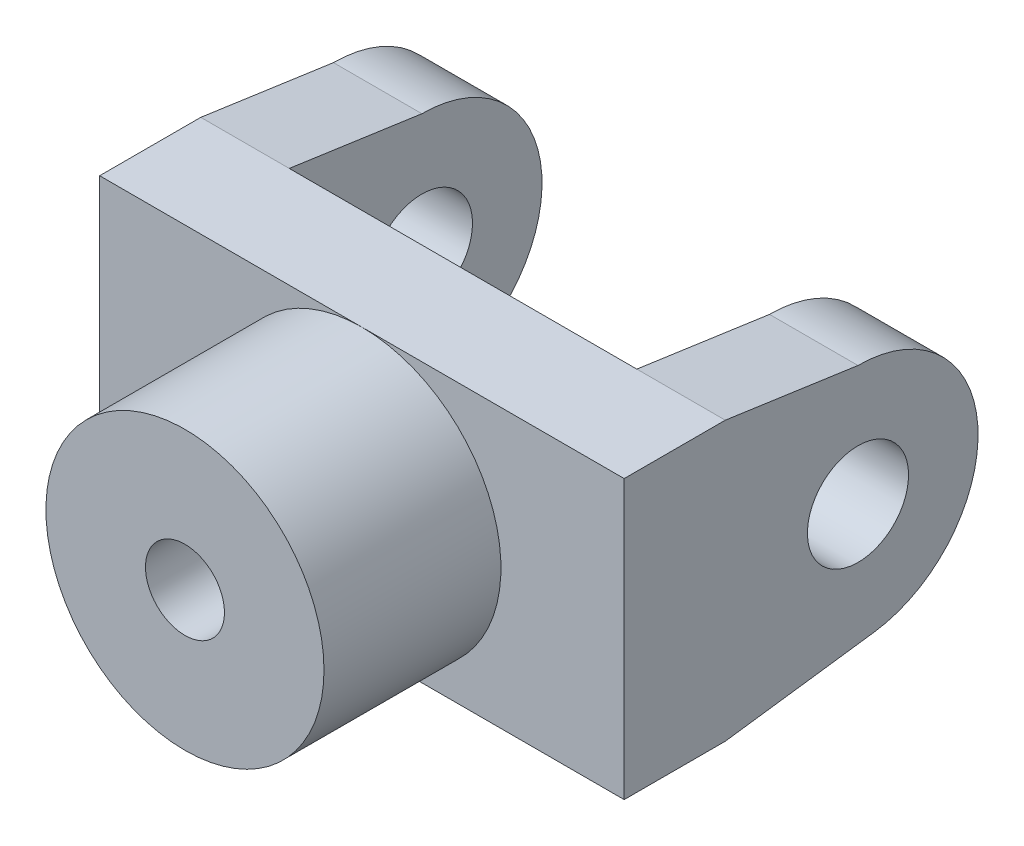
SolidWorks part; units mm, degrees
material "Plain Carbon Steel"
ref_plane "Front Plane" through (0, 0, 0) normal (0, 0, 1) x (1, 0, 0)
ref_plane "Top Plane" through (0, 0, 0) normal (0, 1, 0) x (1, 0, 0)
ref_plane "Right Plane" through (0, 0, 0) normal (1, 0, 0) x (0, 0, -1)
sketch "Base Block Sketch" plane through (0, 0, 0) normal (0, 0, 1) x (1, 0, 0)
  line L1 (83, -44) -> (-83, -44)
  line L2 (83, -44) -> (83, 44)
  line L3 (83, 44) -> (-83, 44)
  line L4 (-83, -44) -> (-83, 44)
  line L5 (83, -44) -> (-83, 44) construction
  line L6 (83, 44) -> (-83, -44) construction
  point P0 (0, 0)
  dimension "D1" = 166
  dimension "D2" = 88
extrude "Base Block 166x88x32" add sketch "Base Block Sketch" along normal blind 32
sketch "Bored Boss Sketch" plane through (0, 0, 32) normal (0, 0, 1) x (1, 0, 0)
  circle A0 centre (0, 0) radius 12.5
  circle A1 centre (0, 0) radius 44
  dimension "D1" = 25
  dimension "D2" = 88
extrude "Bored Boss Ø88 Bore Ø25" add sketch "Bored Boss Sketch" along normal blind 56
sketch "Lug Sketch" plane through (83, 0, 0) normal (1, 0, 0) x (0, 0, -1)
  line L0 (0, 44) -> (0, -44)
  line L1 (0, 0) -> (80, 0) construction
  line L2 (42, 38) -> (0, 44)
  line L3 (0, -44) -> (47.0723, -37.6599)
  arc A0 (47.0723, -37.6599) -> (42, 38) centre (42, 0) ccw
  circle A1 centre (42, 0) radius 16
  dimension "D1" = 32
  dimension "D2" = 76
  dimension "D3" = 42
extrude "Pierced Lug" add sketch "Lug Sketch" against normal blind 28
mirror "Lug Mirror" about plane through (0, 0, 0) normal (1, 0, 0) of "Pierced Lug"
